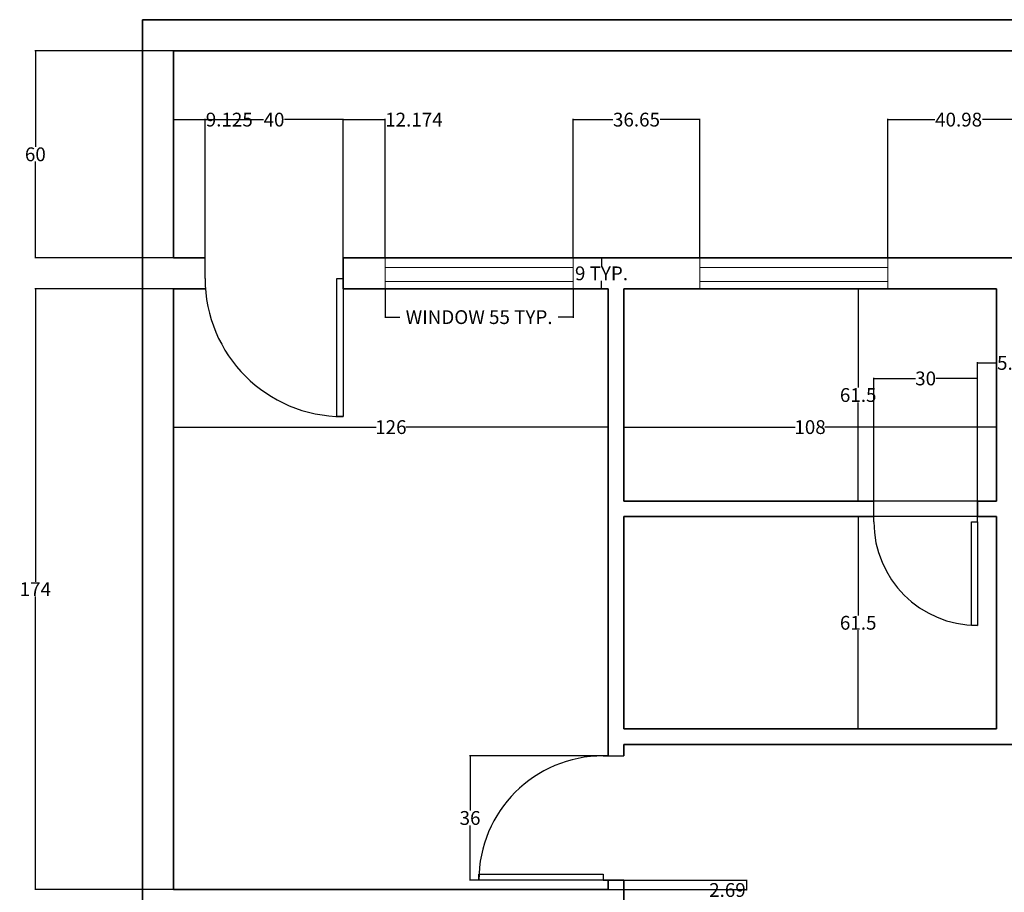
# Model space of a CAD drawing. Units: inches. Extents: x 1353 to 1853, y 16593 to 17433.
# Tile 3 of 4: x 1353 to 1639, y 17180 to 17433. Entities that reach past the tile are written whole.
import ezdxf

# ---------------------------------------------------------------- set-up
doc = ezdxf.new("R2010")
doc.units = ezdxf.units.IN
doc.header["$MEASUREMENT"] = 0
for name, color, linetype, lineweight in [('A-ANNO-DIMS', 2, 'Continuous', 18), ('A-DOOR', 3, 'Continuous', 25), ('A-GLAZ', 4, 'Continuous', 18), ('A-WALL', 7, 'Continuous', 35)]:
    doc.layers.add(name, color=color, linetype=linetype, lineweight=lineweight)
doc.styles.get("Standard").update_dxf_attribs({"font": 'arial.ttf'})
doc.dimstyles.get("Standard").update_dxf_attribs({"dimtxt": 4, "dimasz": 0.18, "dimexe": 0.18, "dimexo": 0.0625, "dimgap": 0.09, "dimtad": 0, "dimtih": 1, "dimtoh": 1, "dimdec": 0, "dimzin": 0, "dimdsep": 46, "dimlunit": 3, "dimtxsty": 'Standard', "dimcen": 0.09, "dimadec": 0, "dimazin": 0, "dimtfac": 1, "dimtdec": 0, "dimtofl": 0, "dimtmove": 0, "dimatfit": 3, "dimfxl": 1, "dimtolj": 1, "dimtzin": 0, "dimarcsym": 0})

# ---------------------------------------------------------------- blocks, each defined once
blk = doc.blocks.new('*U9')
for p, q in [((-40, 0), (-40, 6)), ((0, 0), (0, 6))]:
    blk.add_line(p, q)
blk.add_lwpolyline([(0, 0), (0, -40), (-1.75, -40), (-1.75, 0)], close=True)
blk.add_arc((0, 0), 40, 180, 270)
blk = doc.blocks.new('*U7')
for p, q in [((-30, 0), (-30, 6)), ((0, 0), (0, 6))]:
    blk.add_line(p, q)
blk.add_lwpolyline([(0, 0), (0, -30), (-1.75, -30), (-1.75, 0)], close=True)
blk.add_arc((0, 0), 30, 180, 270)
blk = doc.blocks.new('*U3')
for p, q in [((0, 0), (0, -6)), ((36, 0), (36, -6))]:
    blk.add_line(p, q)
blk.add_lwpolyline([(0, 0), (0, 36), (1.75, 36), (1.75, 0)], close=True)
blk.add_arc((0, 0), 36, 0, 90)
blk = doc.blocks.new('WIN-54_56IN')
for p, q in [((0, 9), (0, 0)), ((54.56, 9), (0, 9)), ((0, 9), (0, 6.2)), ((54.56, 0), (54.56, 9)), ((0, 6.2), (54.56, 6.2)), ((54.56, 6.2), (54.56, 2.15)), ((54.56, 2.15), (0, 2.15))]:
    blk.add_line(p, q)
blk = doc.blocks.new('*D11')
at = {"layer": 'A-ANNO-DIMS', "color": 0, "lineweight": -2, "transparency": 16777216}
for p, q in [((1459.18, 17354.72), (1459.18, 17346.42)), ((1513.74, 17354.72), (1513.74, 17346.42)), ((1459.36, 17346.6), (1463.52, 17346.6)), ((1513.56, 17346.6), (1509.41, 17346.6))]:
    blk.add_line(p, q, dxfattribs=at)
at = {"layer": 'A-ANNO-DIMS', "color": 0, "transparency": 16777216}
for points in [[(1459.36, 17346.63), (1459.36, 17346.57), (1459.18, 17346.6)], [(1513.56, 17346.63), (1513.56, 17346.57), (1513.74, 17346.6)]]:
    blk.add_solid(points, dxfattribs=at)
at = {"layer": 'Defpoints', "color": 0, "transparency": 16777216}
for p in [(1459.18, 17354.78), (1513.74, 17354.78), (1513.74, 17346.6)]:
    blk.add_point(p, dxfattribs=at)
at = {"layer": 'A-ANNO-DIMS', "color": 0, "transparency": 16777216, "insert": (1486.46, 17346.6), "char_height": 4, "attachment_point": 5}
blk.add_mtext('\\A1;WINDOW 55 TYP.', dxfattribs=at)
blk = doc.blocks.new('*D12')
at = {"layer": 'A-ANNO-DIMS', "color": 0, "lineweight": -2, "transparency": 16777216}
for p, q in [((1513.8, 17363.78), (1522.11, 17363.78)), ((1521.93, 17363.6), (1521.93, 17361.41)), ((1513.8, 17354.78), (1522.11, 17354.78)), ((1521.93, 17354.96), (1521.93, 17357.15))]:
    blk.add_line(p, q, dxfattribs=at)
at = {"layer": 'A-ANNO-DIMS', "color": 0, "transparency": 16777216}
for points in [[(1521.9, 17363.6), (1521.96, 17363.6), (1521.93, 17363.78)], [(1521.9, 17354.96), (1521.96, 17354.96), (1521.93, 17354.78)]]:
    blk.add_solid(points, dxfattribs=at)
at = {"layer": 'Defpoints', "color": 0, "transparency": 16777216}
for p in [(1513.74, 17363.78), (1521.93, 17363.78), (1513.74, 17354.78)]:
    blk.add_point(p, dxfattribs=at)
at = {"layer": 'A-ANNO-DIMS', "color": 0, "transparency": 16777216, "insert": (1521.93, 17359.28), "char_height": 4, "attachment_point": 5}
blk.add_mtext('\\A1;9 TYP.', dxfattribs=at)
blk = doc.blocks.new('*D15')
at = {"layer": 'A-ANNO-DIMS', "color": 0, "lineweight": -2, "transparency": 16777216}
for p, q in [((1397.82, 17423.78), (1357.65, 17423.78)), ((1357.83, 17423.6), (1357.83, 17395.91)), ((1357.83, 17363.96), (1357.83, 17391.65)), ((1397.82, 17363.78), (1357.65, 17363.78))]:
    blk.add_line(p, q, dxfattribs=at)
at = {"layer": 'A-ANNO-DIMS', "color": 0, "transparency": 16777216}
for points in [[(1357.8, 17423.6), (1357.86, 17423.6), (1357.83, 17423.78)], [(1357.8, 17363.96), (1357.86, 17363.96), (1357.83, 17363.78)]]:
    blk.add_solid(points, dxfattribs=at)
at = {"layer": 'Defpoints', "color": 0, "transparency": 16777216}
for p in [(1357.83, 17423.78), (1397.88, 17423.78), (1397.88, 17363.78)]:
    blk.add_point(p, dxfattribs=at)
at = {"layer": 'A-ANNO-DIMS', "color": 0, "transparency": 16777216, "insert": (1357.83, 17393.78), "char_height": 4, "attachment_point": 5}
blk.add_mtext('\\A1;60', dxfattribs=at)
blk = doc.blocks.new('*D16')
at = {"layer": 'A-ANNO-DIMS', "color": 0, "lineweight": -2, "transparency": 16777216}
for p, q in [((1397.82, 17354.78), (1357.65, 17354.78)), ((1357.83, 17354.6), (1357.83, 17269.88)), ((1357.83, 17180.96), (1357.83, 17265.68)), ((1397.82, 17180.78), (1357.65, 17180.78))]:
    blk.add_line(p, q, dxfattribs=at)
at = {"layer": 'A-ANNO-DIMS', "color": 0, "transparency": 16777216}
for points in [[(1357.8, 17354.6), (1357.86, 17354.6), (1357.83, 17354.78)], [(1357.8, 17180.96), (1357.86, 17180.96), (1357.83, 17180.78)]]:
    blk.add_solid(points, dxfattribs=at)
at = {"layer": 'Defpoints', "color": 0, "transparency": 16777216}
for p in [(1357.83, 17354.78), (1397.88, 17354.78), (1397.88, 17180.78)]:
    blk.add_point(p, dxfattribs=at)
at = {"layer": 'A-ANNO-DIMS', "color": 0, "transparency": 16777216, "insert": (1357.83, 17267.78), "char_height": 4, "attachment_point": 5}
blk.add_mtext('\\A1;174', dxfattribs=at)
blk = doc.blocks.new('*D23')
at = {"layer": 'A-ANNO-DIMS', "color": 0, "lineweight": -2, "transparency": 16777216}
for p, q in [((1397.88, 17354.72), (1397.88, 17314.55)), ((1523.88, 17354.72), (1523.88, 17314.55)), ((1398.06, 17314.73), (1456.57, 17314.73)), ((1523.7, 17314.73), (1465.2, 17314.73))]:
    blk.add_line(p, q, dxfattribs=at)
at = {"layer": 'A-ANNO-DIMS', "color": 0, "transparency": 16777216}
for points in [[(1398.06, 17314.76), (1398.06, 17314.7), (1397.88, 17314.73)], [(1523.7, 17314.76), (1523.7, 17314.7), (1523.88, 17314.73)]]:
    blk.add_solid(points, dxfattribs=at)
at = {"layer": 'Defpoints', "color": 0, "transparency": 16777216}
for p in [(1397.88, 17354.78), (1523.88, 17354.78), (1397.88, 17314.73)]:
    blk.add_point(p, dxfattribs=at)
at = {"layer": 'A-ANNO-DIMS', "color": 0, "transparency": 16777216, "insert": (1460.88, 17314.73), "char_height": 4, "attachment_point": 5}
blk.add_mtext('\\A1;126', dxfattribs=at)
blk = doc.blocks.new('*D24')
at = {"layer": 'A-ANNO-DIMS', "color": 0, "lineweight": -2, "transparency": 16777216}
for p, q in [((1528.38, 17354.72), (1528.38, 17314.55)), ((1636.38, 17354.72), (1636.38, 17314.55)), ((1528.56, 17314.73), (1578.06, 17314.73)), ((1636.2, 17314.73), (1586.71, 17314.73))]:
    blk.add_line(p, q, dxfattribs=at)
at = {"layer": 'A-ANNO-DIMS', "color": 0, "transparency": 16777216}
for points in [[(1528.56, 17314.76), (1528.56, 17314.7), (1528.38, 17314.73)], [(1636.2, 17314.76), (1636.2, 17314.7), (1636.38, 17314.73)]]:
    blk.add_solid(points, dxfattribs=at)
at = {"layer": 'Defpoints', "color": 0, "transparency": 16777216}
for p in [(1528.38, 17354.78), (1636.38, 17354.78), (1528.38, 17314.73)]:
    blk.add_point(p, dxfattribs=at)
at = {"layer": 'A-ANNO-DIMS', "color": 0, "transparency": 16777216, "insert": (1582.38, 17314.73), "char_height": 4, "attachment_point": 5}
blk.add_mtext('\\A1;108', dxfattribs=at)
blk = doc.blocks.new('*D26')
at = {"layer": 'A-ANNO-DIMS', "color": 0, "lineweight": -2, "transparency": 16777216}
for p, q in [((1636.32, 17354.78), (1596.15, 17354.78)), ((1596.33, 17354.6), (1596.33, 17326.16)), ((1596.33, 17293.46), (1596.33, 17321.9)), ((1636.32, 17293.28), (1596.15, 17293.28))]:
    blk.add_line(p, q, dxfattribs=at)
at = {"layer": 'A-ANNO-DIMS', "color": 0, "transparency": 16777216}
for points in [[(1596.3, 17354.6), (1596.36, 17354.6), (1596.33, 17354.78)], [(1596.3, 17293.46), (1596.36, 17293.46), (1596.33, 17293.28)]]:
    blk.add_solid(points, dxfattribs=at)
at = {"layer": 'Defpoints', "color": 0, "transparency": 16777216}
for p in [(1596.33, 17354.78), (1636.38, 17354.78), (1636.38, 17293.28)]:
    blk.add_point(p, dxfattribs=at)
at = {"layer": 'A-ANNO-DIMS', "color": 0, "transparency": 16777216, "insert": (1596.33, 17324.03), "char_height": 4, "attachment_point": 5}
blk.add_mtext('\\A1;61.5', dxfattribs=at)
blk = doc.blocks.new('*D27')
at = {"layer": 'A-ANNO-DIMS', "color": 0, "lineweight": -2, "transparency": 16777216}
for p, q in [((1636.32, 17288.78), (1596.15, 17288.78)), ((1596.33, 17288.6), (1596.33, 17260.16)), ((1596.33, 17227.46), (1596.33, 17255.9)), ((1636.32, 17227.28), (1596.15, 17227.28))]:
    blk.add_line(p, q, dxfattribs=at)
at = {"layer": 'A-ANNO-DIMS', "color": 0, "transparency": 16777216}
for points in [[(1596.3, 17288.6), (1596.36, 17288.6), (1596.33, 17288.78)], [(1596.3, 17227.46), (1596.36, 17227.46), (1596.33, 17227.28)]]:
    blk.add_solid(points, dxfattribs=at)
at = {"layer": 'Defpoints', "color": 0, "transparency": 16777216}
for p in [(1596.33, 17288.78), (1636.38, 17288.78), (1636.38, 17227.28)]:
    blk.add_point(p, dxfattribs=at)
at = {"layer": 'A-ANNO-DIMS', "color": 0, "transparency": 16777216, "insert": (1596.33, 17258.03), "char_height": 4, "attachment_point": 5}
blk.add_mtext('\\A1;61.5', dxfattribs=at)
blk = doc.blocks.new('*D34')
at = {"layer": 'A-ANNO-DIMS', "color": 0, "lineweight": -2, "transparency": 16777216}
for p, q in [((1407.01, 17363.84), (1407.01, 17404.01)), ((1407.19, 17403.83), (1423.98, 17403.83)), ((1446.83, 17403.83), (1430.04, 17403.83)), ((1447.01, 17363.84), (1447.01, 17404.01))]:
    blk.add_line(p, q, dxfattribs=at)
at = {"layer": 'A-ANNO-DIMS', "color": 0, "transparency": 16777216}
for points in [[(1407.19, 17403.86), (1407.19, 17403.8), (1407.01, 17403.83)], [(1446.83, 17403.86), (1446.83, 17403.8), (1447.01, 17403.83)]]:
    blk.add_solid(points, dxfattribs=at)
at = {"layer": 'Defpoints', "color": 0, "transparency": 16777216}
for p in [(1447.01, 17403.83), (1407.01, 17363.78), (1447.01, 17363.78)]:
    blk.add_point(p, dxfattribs=at)
at = {"layer": 'A-ANNO-DIMS', "color": 0, "transparency": 16777216, "insert": (1427.01, 17403.83), "char_height": 4, "attachment_point": 5}
blk.add_mtext('\\A1;40', dxfattribs=at)
blk = doc.blocks.new('*D37')
at = {"layer": 'A-ANNO-DIMS', "color": 0, "lineweight": -2, "transparency": 16777216}
for p, q in [((1397.88, 17363.84), (1397.88, 17404.01)), ((1398.06, 17403.83), (1406.83, 17403.83)), ((1407.01, 17363.84), (1407.01, 17404.01)), ((1407.01, 17403.83), (1407.19, 17403.83))]:
    blk.add_line(p, q, dxfattribs=at)
at = {"layer": 'A-ANNO-DIMS', "color": 0, "transparency": 16777216}
for points in [[(1398.06, 17403.86), (1398.06, 17403.8), (1397.88, 17403.83)], [(1406.83, 17403.86), (1406.83, 17403.8), (1407.01, 17403.83)]]:
    blk.add_solid(points, dxfattribs=at)
at = {"layer": 'Defpoints', "color": 0, "transparency": 16777216}
for p in [(1407.01, 17403.83), (1397.88, 17363.78), (1407.01, 17363.78)]:
    blk.add_point(p, dxfattribs=at)
at = {"layer": 'A-ANNO-DIMS', "color": 0, "transparency": 16777216, "insert": (1414.04, 17403.83), "char_height": 4, "attachment_point": 5}
blk.add_mtext('\\A1;9.125', dxfattribs=at)
blk = doc.blocks.new('*D38')
at = {"layer": 'A-ANNO-DIMS', "color": 0, "lineweight": -2, "transparency": 16777216}
for p, q in [((1447.009276, 17363.843389), (1447.009276, 17404.010889)), ((1447.189276, 17403.830889), (1459.002956, 17403.830889)), ((1459.182956, 17363.843389), (1459.182956, 17404.010889)), ((1459.182956, 17403.830889), (1459.362956, 17403.830889))]:
    blk.add_line(p, q, dxfattribs=at)
at = {"layer": 'A-ANNO-DIMS', "color": 0, "transparency": 16777216}
for points in [[(1447.189276, 17403.860889), (1447.189276, 17403.800889), (1447.009276, 17403.830889)], [(1459.002956, 17403.860889), (1459.002956, 17403.800889), (1459.182956, 17403.830889)]]:
    blk.add_solid(points, dxfattribs=at)
at = {"layer": 'Defpoints', "color": 0, "transparency": 16777216}
for p in [(1459.182956, 17403.830889), (1447.009276, 17363.780889), (1459.182956, 17363.780889)]:
    blk.add_point(p, dxfattribs=at)
at = {"layer": 'A-ANNO-DIMS', "color": 0, "transparency": 16777216, "insert": (1467.559368, 17403.830889), "char_height": 4, "attachment_point": 5}
blk.add_mtext('\\A1;12.174', dxfattribs=at)
blk = doc.blocks.new('*D39')
at = {"layer": 'A-ANNO-DIMS', "color": 0, "lineweight": -2, "transparency": 16777216}
for p, q in [((1513.74, 17363.84), (1513.74, 17404.01)), ((1513.92, 17403.83), (1525.21, 17403.83)), ((1550.21, 17403.83), (1538.92, 17403.83)), ((1550.39, 17363.84), (1550.39, 17404.01))]:
    blk.add_line(p, q, dxfattribs=at)
at = {"layer": 'A-ANNO-DIMS', "color": 0, "transparency": 16777216}
for points in [[(1513.92, 17403.86), (1513.92, 17403.8), (1513.74, 17403.83)], [(1550.21, 17403.86), (1550.21, 17403.8), (1550.39, 17403.83)]]:
    blk.add_solid(points, dxfattribs=at)
at = {"layer": 'Defpoints', "color": 0, "transparency": 16777216}
for p in [(1550.39, 17403.83), (1513.74, 17363.78), (1550.39, 17363.78)]:
    blk.add_point(p, dxfattribs=at)
at = {"layer": 'A-ANNO-DIMS', "color": 0, "transparency": 16777216, "insert": (1532.07, 17403.83), "char_height": 4, "attachment_point": 5}
blk.add_mtext('\\A1;36.65', dxfattribs=at)
blk = doc.blocks.new('*D40')
at = {"layer": 'A-ANNO-DIMS', "color": 0, "lineweight": -2, "transparency": 16777216}
for p, q in [((1604.95, 17363.84), (1604.95, 17404.01)), ((1605.13, 17403.83), (1618.52, 17403.83)), ((1645.75, 17403.83), (1632.36, 17403.83)), ((1645.93, 17363.84), (1645.93, 17404.01))]:
    blk.add_line(p, q, dxfattribs=at)
at = {"layer": 'A-ANNO-DIMS', "color": 0, "transparency": 16777216}
for points in [[(1605.13, 17403.86), (1605.13, 17403.8), (1604.95, 17403.83)], [(1645.75, 17403.86), (1645.75, 17403.8), (1645.93, 17403.83)]]:
    blk.add_solid(points, dxfattribs=at)
at = {"layer": 'Defpoints', "color": 0, "transparency": 16777216}
for p in [(1645.93, 17403.83), (1604.95, 17363.78), (1645.93, 17363.78)]:
    blk.add_point(p, dxfattribs=at)
at = {"layer": 'A-ANNO-DIMS', "color": 0, "transparency": 16777216, "insert": (1625.44, 17403.83), "char_height": 4, "attachment_point": 5}
blk.add_mtext('\\A1;40.98', dxfattribs=at)
blk = doc.blocks.new('*D51')
at = {"layer": 'A-ANNO-DIMS', "color": 0, "lineweight": -2, "transparency": 16777216}
for p, q in [((1600.88, 17288.84), (1600.88, 17329.01)), ((1601.06, 17328.83), (1612.93, 17328.83)), ((1630.7, 17328.83), (1618.82, 17328.83)), ((1630.88, 17288.84), (1630.88, 17329.01))]:
    blk.add_line(p, q, dxfattribs=at)
at = {"layer": 'A-ANNO-DIMS', "color": 0, "transparency": 16777216}
for points in [[(1601.06, 17328.86), (1601.06, 17328.8), (1600.88, 17328.83)], [(1630.7, 17328.86), (1630.7, 17328.8), (1630.88, 17328.83)]]:
    blk.add_solid(points, dxfattribs=at)
at = {"layer": 'Defpoints', "color": 0, "transparency": 16777216}
for p in [(1630.88, 17328.83), (1600.88, 17288.78), (1630.88, 17288.78)]:
    blk.add_point(p, dxfattribs=at)
at = {"layer": 'A-ANNO-DIMS', "color": 0, "transparency": 16777216, "insert": (1615.88, 17328.83), "char_height": 4, "attachment_point": 5}
blk.add_mtext('\\A1;30', dxfattribs=at)
blk = doc.blocks.new('*D52')
at = {"layer": 'A-ANNO-DIMS', "color": 0, "lineweight": -2, "transparency": 16777216}
for p, q in [((1630.88, 17293.34), (1630.88, 17333.51)), ((1631.06, 17333.33), (1636.2, 17333.33)), ((1636.38, 17293.34), (1636.38, 17333.51)), ((1636.38, 17333.33), (1636.56, 17333.33))]:
    blk.add_line(p, q, dxfattribs=at)
at = {"layer": 'A-ANNO-DIMS', "color": 0, "transparency": 16777216}
for points in [[(1631.06, 17333.36), (1631.06, 17333.3), (1630.88, 17333.33)], [(1636.2, 17333.36), (1636.2, 17333.3), (1636.38, 17333.33)]]:
    blk.add_solid(points, dxfattribs=at)
at = {"layer": 'Defpoints', "color": 0, "transparency": 16777216}
for p in [(1636.38, 17333.33), (1630.88, 17293.28), (1636.38, 17293.28)]:
    blk.add_point(p, dxfattribs=at)
at = {"layer": 'A-ANNO-DIMS', "color": 0, "transparency": 16777216, "insert": (1643.4, 17333.33), "char_height": 4, "attachment_point": 5}
blk.add_mtext('\\A1;5.506', dxfattribs=at)
blk = doc.blocks.new('*D55')
at = {"layer": 'A-ANNO-DIMS', "color": 0, "lineweight": -2, "transparency": 16777216}
for p, q in [((1523.82, 17219.47), (1483.65, 17219.47)), ((1483.83, 17219.29), (1483.83, 17203.6)), ((1483.83, 17183.65), (1483.83, 17199.33)), ((1523.82, 17183.47), (1483.65, 17183.47))]:
    blk.add_line(p, q, dxfattribs=at)
at = {"layer": 'A-ANNO-DIMS', "color": 0, "transparency": 16777216}
for points in [[(1483.8, 17219.29), (1483.86, 17219.29), (1483.83, 17219.47)], [(1483.8, 17183.65), (1483.86, 17183.65), (1483.83, 17183.47)]]:
    blk.add_solid(points, dxfattribs=at)
at = {"layer": 'Defpoints', "color": 0, "transparency": 16777216}
for p in [(1483.83, 17219.47), (1523.88, 17219.47), (1523.88, 17183.47)]:
    blk.add_point(p, dxfattribs=at)
at = {"layer": 'A-ANNO-DIMS', "color": 0, "transparency": 16777216, "insert": (1483.83, 17201.47), "char_height": 4, "attachment_point": 5}
blk.add_mtext('\\A1;36', dxfattribs=at)
blk = doc.blocks.new('*D56')
at = {"layer": 'A-ANNO-DIMS', "color": 0, "lineweight": -2, "transparency": 16777216}
for p, q in [((1523.95, 17183.47), (1564.11, 17183.47)), ((1523.95, 17180.78), (1564.11, 17180.78)), ((1563.93, 17183.29), (1563.93, 17180.96)), ((1563.93, 17180.78), (1563.93, 17180.6)), ((1563.93, 17180.6), (1563.75, 17180.6))]:
    blk.add_line(p, q, dxfattribs=at)
at = {"layer": 'A-ANNO-DIMS', "color": 0, "transparency": 16777216}
for points in [[(1563.9, 17183.29), (1563.96, 17183.29), (1563.93, 17183.47)], [(1563.9, 17180.96), (1563.96, 17180.96), (1563.93, 17180.78)]]:
    blk.add_solid(points, dxfattribs=at)
at = {"layer": 'Defpoints', "color": 0, "transparency": 16777216}
for p in [(1523.88, 17183.47), (1523.88, 17180.78), (1563.93, 17180.78)]:
    blk.add_point(p, dxfattribs=at)
at = {"layer": 'A-ANNO-DIMS', "color": 0, "transparency": 16777216, "insert": (1558.43, 17180.6), "char_height": 4, "attachment_point": 5}
blk.add_mtext('\\A1;2.69', dxfattribs=at)

msp = doc.modelspace()

# ---------------------------------------------------------------- linework, layer by layer
at = {"layer": 'A-WALL'}
for p, q in [((1388.8844, 17432.7809), (1808.8844, 17432.7809)), ((1388.8844, 16635.7809), (1388.8844, 17432.7809)), ((1397.8844, 17423.7809), (1799.8844, 17423.7809)), ((1397.8844, 17363.7809), (1397.8844, 17423.7809)), ((1397.8844, 17363.7809), (1400.0526, 17363.7809)), ((1398.9685, 17363.7809), (1407.0093, 17363.7809)), ((1400.0526, 17363.7809), (1400.0526, 17363.7809)), ((1447.0093, 17354.7809), (1447.0093, 17363.7809)), ((1459.183, 17363.7809), (1447.0093, 17363.7809)), ((1459.183, 17363.7809), (1645.9302, 17363.7809)), ((1397.8844, 17354.7809), (1400.0526, 17354.7809)), ((1397.8844, 17180.7809), (1397.8844, 17354.7809)), ((1400.0526, 17354.7809), (1407.1219, 17354.7809)), ((1459.183, 17354.7809), (1447.0093, 17354.7809)), ((1459.183, 17354.7809), (1523.8844, 17354.7809)), ((1523.8844, 17219.4674), (1523.8844, 17354.7809)), ((1528.3844, 17293.2809), (1528.3844, 17354.7809)), ((1528.3844, 17354.7809), (1636.3844, 17354.7809)), ((1636.3844, 17293.2809), (1636.3844, 17354.7809)), ((1528.3844, 17293.2809), (1600.8782, 17293.2809)), ((1600.8782, 17293.2809), (1586.1354, 17293.2809)), ((1599.7933, 17293.2809), (1600.8782, 17293.2809)), ((1630.8782, 17288.7809), (1630.8782, 17293.2809)), ((1630.8782, 17293.2809), (1636.3844, 17293.2809)), ((1528.3844, 17288.7809), (1600.8782, 17288.7809)), ((1528.3844, 17227.2809), (1528.3844, 17288.7809)), ((1586.1354, 17288.7809), (1600.8782, 17288.7809)), ((1630.8782, 17288.7809), (1636.3844, 17288.7809)), ((1636.3844, 17227.2809), (1636.3844, 17288.7809)), ((1528.3844, 17227.2809), (1636.3844, 17227.2809)), ((1528.3844, 17222.7809), (1640.9844, 17222.7809)), ((1528.3844, 17219.4674), (1528.3844, 17222.7809)), ((1397.8844, 17180.7809), (1422.0272, 17180.7809)), ((1420.6798, 17180.7809), (1455.9979, 17180.7809)), ((1455.9979, 17180.7809), (1523.8844, 17180.7809)), ((1523.8844, 17180.7809), (1523.8844, 17183.4674)), ((1523.8844, 17183.4674), (1528.3844, 17183.4674)), ((1528.3844, 17176.2809), (1528.3844, 17183.4674))]:
    msp.add_line(p, q, dxfattribs=at)

# ---------------------------------------------------------------- block references
at = {"layer": 'A-DOOR'}
for name, p in [('*U9', (1447.0093, 17357.7809)), ('*U7', (1630.8782, 17287.2809))]:
    msp.add_blockref(name, p, dxfattribs=at)
at = {"layer": 'A-DOOR', "rotation": 90}
msp.add_blockref('*U3', (1522.3852, 17183.4674), dxfattribs=at)
at = {"layer": 'A-GLAZ'}
for p in [(1459.183, 17354.781), (1550.3928, 17354.781), (1550.3928, 17354.781)]:
    msp.add_blockref('WIN-54_56IN', p, dxfattribs=at)

# ---------------------------------------------------------------- dimensions: what is measured, and where the dimension line sits
at = {"layer": 'A-ANNO-DIMS'}
for base, p1, p2, angle, override, picture, middle in [((1357.8344, 17423.7809), (1397.8844, 17363.7809), (1397.8844, 17423.7809), 90, {"dimdec": 0, "dimlfac": 1, "dimrnd": 0, "dimzin": 0, "dimdsep": 46, "dimlunit": 2}, '*D15', (1357.8344, 17393.7809)), ((1357.8344, 17354.7809), (1397.8844, 17180.7809), (1397.8844, 17354.7809), 90, {"dimdec": 0, "dimlfac": 1, "dimrnd": 0, "dimzin": 0, "dimdsep": 46, "dimlunit": 2}, '*D16', (1357.8344, 17267.7809)), ((1397.8844, 17314.7309), (1523.8844, 17354.7809), (1397.8844, 17354.7809), 180, {"dimdec": 0, "dimlfac": 1, "dimrnd": 0, "dimzin": 0, "dimdsep": 46, "dimlunit": 2}, '*D23', (1460.8844, 17314.7309)), ((1528.3844, 17314.7309), (1636.3844, 17354.7809), (1528.3844, 17354.7809), 180, {"dimdec": 0, "dimlfac": 1, "dimrnd": 0, "dimzin": 0, "dimdsep": 46, "dimlunit": 2}, '*D24', (1582.3844, 17314.7309)), ((1596.3344, 17354.7809), (1636.3844, 17293.2809), (1636.3844, 17354.7809), 90, {"dimdec": 1, "dimlfac": 1, "dimrnd": 0, "dimzin": 0, "dimdsep": 46, "dimlunit": 2}, '*D26', (1596.3344, 17324.0309)), ((1596.3344, 17288.7809), (1636.3844, 17227.2809), (1636.3844, 17288.7809), 90, {"dimdec": 1, "dimlfac": 1, "dimrnd": 0, "dimzin": 0, "dimdsep": 46, "dimlunit": 2}, '*D27', (1596.3344, 17258.0309)), ((1483.8344, 17219.4674), (1523.8844, 17183.4674), (1523.8844, 17219.4674), 90, {"dimdec": 0, "dimlfac": 1, "dimrnd": 0, "dimzin": 0, "dimdsep": 46, "dimlunit": 2}, '*D55', (1483.8344, 17201.4674)), ((1563.9344, 17180.7809), (1523.8844, 17183.4674), (1523.8844, 17180.7809), 270, {"dimdec": 2, "dimlfac": 1, "dimrnd": 0, "dimzin": 0, "dimdsep": 46, "dimlunit": 2}, '*D56', (1558.4311, 17180.6009))]:
    dim = msp.add_linear_dim(base=base, p1=p1, p2=p2, angle=angle, dimstyle='Standard', override=override, dxfattribs=at)
    dim.commit()
    dim.dimension.update_dxf_attribs({"geometry": picture, "text_midpoint": middle})
for base, p1, p2, override, picture, middle in [((1407.0093, 17403.8309), (1397.8844, 17363.7809), (1407.0093, 17363.7809), {"dimdec": 3, "dimlfac": 1, "dimrnd": 0, "dimzin": 0, "dimdsep": 46, "dimlunit": 2}, '*D37', (1414.0433, 17403.8309)), ((1447.0093, 17403.8309), (1407.0093, 17363.7809), (1447.0093, 17363.7809), {"dimdec": 0, "dimlfac": 1, "dimrnd": 0, "dimzin": 0, "dimdsep": 46, "dimlunit": 2}, '*D34', (1427.0093, 17403.8309)), ((1459.183, 17403.8309), (1447.0093, 17363.7809), (1459.183, 17363.7809), {"dimdec": 3, "dimlfac": 1, "dimrnd": 0, "dimzin": 0, "dimdsep": 46, "dimlunit": 2}, '*D38', (1467.5594, 17403.8309)), ((1550.3928, 17403.8309), (1513.7424, 17363.7809), (1550.3928, 17363.7809), {"dimdec": 2, "dimlfac": 1, "dimrnd": 0, "dimzin": 0, "dimdsep": 46, "dimlunit": 2}, '*D39', (1532.0676, 17403.8309)), ((1645.9302, 17403.8309), (1604.9522, 17363.7809), (1645.9302, 17363.7809), {"dimdec": 2, "dimlfac": 1, "dimrnd": 0, "dimzin": 0, "dimdsep": 46, "dimlunit": 2}, '*D40', (1625.4412, 17403.8309)), ((1636.3844, 17333.3309), (1630.8782, 17293.2809), (1636.3844, 17293.2809), {"dimdec": 3, "dimlfac": 1, "dimrnd": 0, "dimzin": 0, "dimdsep": 46, "dimlunit": 2}, '*D52', (1643.402, 17333.3309)), ((1630.8782, 17328.8309), (1600.8782, 17288.7809), (1630.8782, 17288.7809), {"dimdec": 0, "dimlfac": 1, "dimrnd": 0, "dimzin": 0, "dimdsep": 46, "dimlunit": 2}, '*D51', (1615.8782, 17328.8309))]:
    dim = msp.add_linear_dim(base=base, p1=p1, p2=p2, dimstyle='Standard', override=override, dxfattribs=at)
    dim.commit()
    dim.dimension.update_dxf_attribs({"geometry": picture, "text_midpoint": middle})
dim = msp.add_linear_dim(base=(1521.9263, 17363.7809), p1=(1513.7424, 17354.7809), p2=(1513.7424, 17363.7809), angle=90, text='<> TYP.', dimstyle='Standard', override={"dimdec": 0, "dimlfac": 1, "dimrnd": 0, "dimzin": 0, "dimdsep": 46, "dimlunit": 2}, dxfattribs=at)
dim.commit()
dim.dimension.update_dxf_attribs({"geometry": '*D12', "text_midpoint": (1521.9263, 17359.2809)})
dim = msp.add_linear_dim(base=(1513.7424, 17346.597), p1=(1459.183, 17354.7809), p2=(1513.7424, 17354.7809), text='WINDOW <> TYP.', dimstyle='Standard', override={"dimdec": 0, "dimlfac": 1, "dimrnd": 0, "dimzin": 0, "dimdsep": 46, "dimlunit": 2}, dxfattribs=at)
dim.commit()
dim.dimension.update_dxf_attribs({"geometry": '*D11', "text_midpoint": (1486.4627, 17346.597)})

doc.saveas('drawing.dxf')
